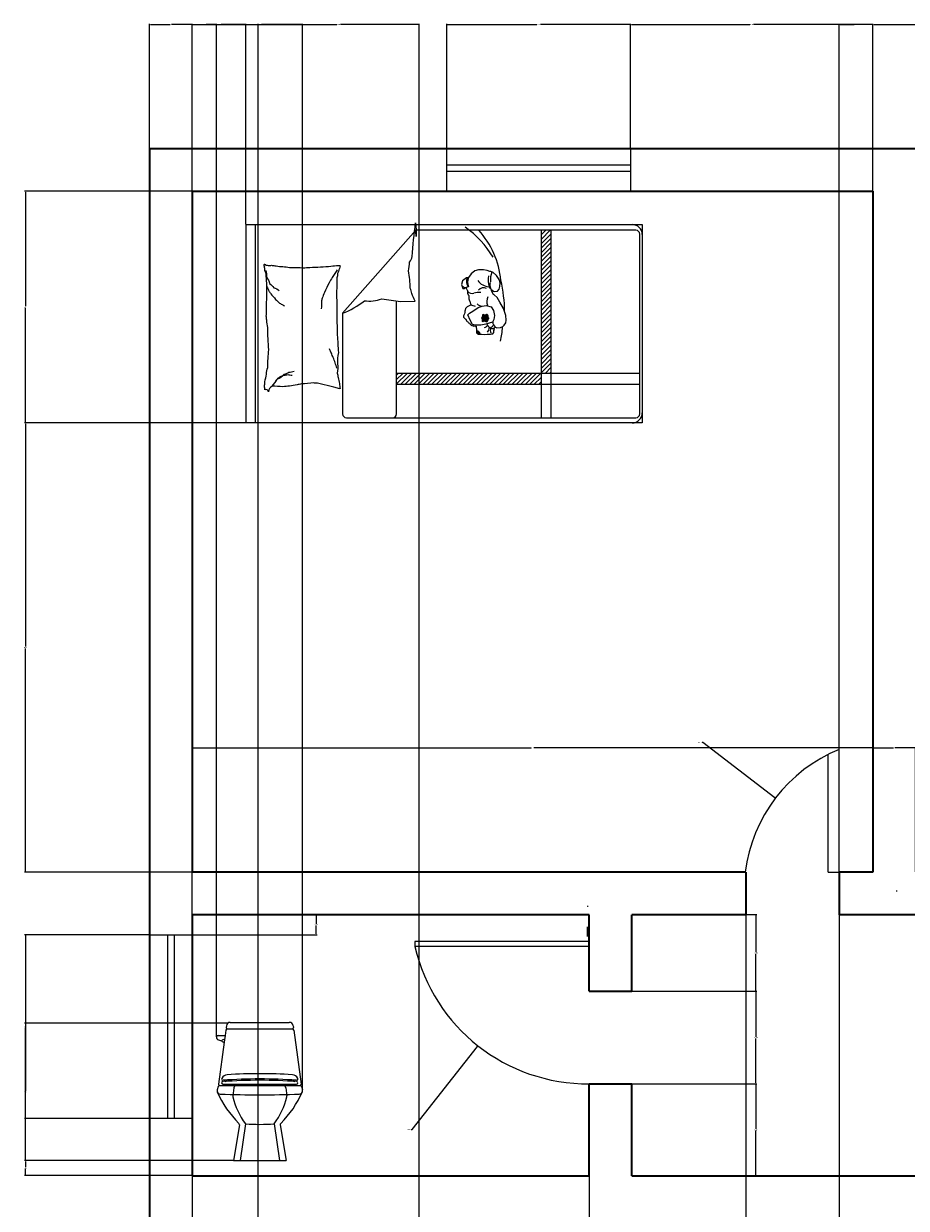
# Model space of a CAD drawing. Units: inches. Extents: x -20 to 351, y -512 to 63.
# Tile 4 of 5: x -20 to 166, y -188 to 63. Entities that reach past the tile are written whole.
import ezdxf

# ---------------------------------------------------------------- set-up
doc = ezdxf.new("R2010")
doc.units = ezdxf.units.IN
doc.header["$MEASUREMENT"] = 0
for name, color, linetype, lineweight in [('A-ANNO-DIMS', 2, 'Continuous', 18), ('A-DOOR', 3, 'Continuous', 18), ('A-FURN', 30, 'Continuous', 18), ('A-GLAZ', 4, 'Continuous', 18), ('A-WALL', 7, 'Continuous', 35), ('WC-Detail_dwgmodels.com', 31, 'Continuous', 13), ('WC-Outline_dwgmodels.com', 31, 'Continuous', 18)]:
    doc.layers.add(name, color=color, linetype=linetype, lineweight=lineweight)
doc.styles.get("Standard").update_dxf_attribs({"font": 'arial.ttf'})
doc.dimstyles.get("Standard").update_dxf_attribs({"dimtxt": 0.18, "dimasz": 0.18, "dimexe": 0.18, "dimexo": 0.0625, "dimgap": 0.09, "dimtad": 0, "dimtih": 1, "dimtoh": 1, "dimdec": 4, "dimzin": 0, "dimdsep": 46, "dimtxsty": 'Standard', "dimcen": 0.09, "dimadec": 0, "dimazin": 0, "dimtfac": 1, "dimtdec": 4, "dimtofl": 0, "dimtmove": 0, "dimatfit": 3, "dimfxl": 1, "dimtolj": 1, "dimtzin": 0, "dimarcsym": 0})
pattern_1 = [(135, (-420.77409, 493.76136), (-0.08072188, -0.08072188), [])]

# ---------------------------------------------------------------- blocks, each defined once
blk = doc.blocks.new('BED-SINGLE')
h = blk.add_hatch()
h.set_pattern_fill('ANSI31', color=256, scale=0.209657, angle=90, style=0)
h.set_pattern_definition([(225, (-28.8794, 49.6857), (-0.4706923, 0.4706923), [])])
h.paths.add_polyline_path([(62.56, 8.11), (62.56, 10.46), (31.92, 10.46), (31.92, 8.11)])
h.paths.add_polyline_path([(64.62, 10.46), (64.62, 40.74), (62.56, 40.74), (62.56, 10.46)])
h = blk.add_hatch()
h.set_pattern_fill('ANSI31', color=256, scale=0.913264, angle=90, style=0)
h.set_pattern_definition(pattern_1)
h.paths.add_polyline_path([(51.28, 22.35), (51.3, 22.58), (51.22, 22.8), (51.07, 22.92), (50.9, 22.92), (50.65, 22.81), (50.46, 22.77), (50.38, 22.84), (50.26, 22.89), (50.12, 22.84), (50.1, 22.73), (50.1, 22.6), (50.04, 22.43), (49.91, 22.22), (49.88, 22.16), (50.03, 21.91), (50.07, 21.8), (50.04, 21.63), (50.02, 21.51), (50.13, 21.39), (50.25, 21.43), (50.34, 21.55), (50.56, 21.53), (50.93, 21.38), (51.11, 21.41), (51.13, 21.53), (51.16, 21.62), (51.25, 21.7), (51.25, 21.79), (51.3, 21.95), (51.4, 22.06), (51.46, 22.11), (51.37, 22.18)])
h = blk.add_hatch()
h.set_pattern_fill('ANSI31', color=256, scale=0.913264, angle=90, style=0)
h.set_pattern_definition(pattern_1)
h.paths.add_polyline_path([(48.8, 19.38), (48.81, 19.17), (48.88, 18.99), (49.05, 18.85), (49.19, 18.79), (49.55, 18.75, 0.479357)])
for p, q in [((0, 41.93), (83.86, 41.93)), ((20.48, 23.17), (35.99, 40.74)), ((82.51, 40.74), (35.99, 40.74)), ((62.56, 1.08), (62.56, 40.74)), ((64.62, 1.08), (64.62, 40.74)), ((83.86, 41.93), (83.86, 0)), ((83.35, 1.92), (83.35, 39.9)), ((31.92, 1.92), (31.92, 25.76)), ((20.48, 23.17), (20.48, 1.92)), ((83.86, 0), (0, 0)), ((21.32, 1.08), (82.51, 1.08))]:
    blk.add_line(p, q)
for points in [[(0, 41.93), (0, 0)], [(2.1, 0), (2.1, 41.93)], [(49.88, 18.74), (50.44, 18.72), (51.09, 18.75), (51.78, 18.78), (51.99, 18.81), (52.24, 18.82), (52.5, 19.09), (52.51, 19.35), (52.46, 19.55), (52.59, 19.75), (52.54, 19.93), (52.68, 20.27), (52.85, 20.24), (53.09, 20.11), (53.92, 20.14), (54.4, 20.39), (54.7, 20.65), (55.03, 21.16), (55.11, 21.69), (54.99, 22.73), (54.51, 24.21), (53.78, 25.53), (53.17, 26.52), (52.53, 27.05), (52.38, 27.16), (51.98, 27.94), (51.97, 28.02), (52.04, 28.1), (52.44, 27.84), (52.72, 27.76), (53.28, 27.82), (53.58, 28.27), (53.78, 28.87), (53.81, 29.61), (53.61, 30.34), (53.08, 31.16), (52.32, 31.81), (51.86, 31.98), (51.61, 32), (51.05, 32.23), (50.29, 32.34), (49.27, 32.34), (48.48, 32.12), (47.69, 31.5), (47.1, 30.74), (46.7, 30.65), (45.83, 30.03), (45.63, 29.27), (45.94, 28.45), (46.23, 28.39), (46.51, 28.63), (46.59, 28.65), (46.7, 28.38), (46.79, 28.19), (46.84, 28.15), (46.88, 27.91), (46.94, 27.83), (46.9, 27.43), (47.08, 27.07), (47.21, 26.95), (47.22, 26.46), (47.16, 26.24), (47.34, 25.81), (47.42, 25.77), (47.46, 25.38), (47.62, 25.1), (47.53, 24.92), (47.25, 24.78), (46.82, 24.56), (46.52, 24.21), (46.42, 23.85), (46.36, 23.64), (46.33, 23.32), (46.29, 23.08), (46.15, 22.79), (46.09, 22.63), (46.1, 22.34), (46.39, 21.98), (46.55, 21.94), (46.69, 21.61), (46.82, 21.43), (46.98, 21.37), (47.06, 21.28), (47.13, 21.18), (47.37, 21.06), (47.42, 21.02), (47.42, 20.94), (47.65, 20.72), (47.76, 20.61), (47.94, 20.63), (48.13, 20.48), (48.29, 20.49), (48.59, 20.46), (48.72, 20.43), (48.78, 20.4), (48.76, 20.33), (48.74, 20.13), (48.82, 19.97), (48.83, 19.89), (48.79, 19.52), (48.81, 19.17), (48.88, 18.99), (49.05, 18.85), (49.19, 18.79), (49.73, 18.74), (49.88, 18.74)], [(47.98, 20.81), (47.46, 21.73), (46.99, 22.87), (47.37, 23.23), (48.03, 23.64), (49.19, 24.37), (50.01, 24.7), (50.89, 24.79), (51.92, 24.54), (52.4, 23.78), (52.6, 22.7), (52.51, 21.89), (52.18, 21.31), (50.82, 20.9), (49.74, 20.66), (48.6, 20.63), (47.98, 20.81)], [(49.88, 22.16), (50.03, 21.91), (50.07, 21.8), (50.04, 21.63), (50.02, 21.51), (50.13, 21.39), (50.25, 21.43), (50.34, 21.55), (50.56, 21.53), (50.93, 21.38), (51.11, 21.41), (51.13, 21.53), (51.16, 21.62), (51.25, 21.7), (51.25, 21.79), (51.3, 21.95), (51.4, 22.06), (51.46, 22.11), (51.37, 22.18), (51.28, 22.35), (51.3, 22.58), (51.22, 22.8), (51.07, 22.92), (50.9, 22.92), (50.65, 22.81), (50.46, 22.77), (50.38, 22.84), (50.26, 22.89), (50.12, 22.84), (50.1, 22.73), (50.1, 22.6), (50.04, 22.43), (49.91, 22.22), (49.88, 22.16)], [(83.35, 10.46), (31.92, 10.46)], [(83.35, 8.11), (31.92, 8.11)]]:
    blk.add_lwpolyline(points)
for points in [[(35.81, 25.72, 0.027362), (35.12, 27.33, 0.040834), (34.81, 28.47, 0.038441), (34.42, 32.14, 0.076528), (34.64, 34, 0.103649), (35.24, 35.15, -0.018778), (35.94, 42.28, -0.024037), (36.09, 39.44, -0.052315), (35.99, 40.74)], [(5.6, 7.76, 0.263368), (4.81, 6.59, 0.494818), (4.03, 6.97, 0.049225), (3.96, 7.71, 0.036831), (4.03, 8.71, 0.031893), (4.37, 10.3, -0.035782), (4.66, 11.72, -0.032941), (4.91, 15.48, -0.026564), (4.66, 20.14, -0.017905), (4.44, 21.72, 0.033397), (4.34, 22.56, 0.03204), (4.37, 24.12, -0.018442), (4.5, 26.82, -0.010837), (4.47, 29.53, -0.014624), (4.34, 31.54, -0.111249), (4.04, 32.49, 0.153708), (3.87, 33.19, 0.076444), (3.94, 33.51, 0.215512), (4.03, 33.59, 0.585858), (4.16, 33.48, -0.363489), (4.26, 33.27, -0.191716), (4.75, 33.27, 0.129675), (5.45, 33.35, 0.01735), (6.15, 33.23, -0.019326), (6.78, 33.12, -0.018818), (9.65, 32.84, -0.021828), (12.13, 32.8, -0.006204), (13.55, 32.86, -0.001963), (18.04, 33.12, -0.028341), (19.55, 33.29, 0.117014), (19.92, 33.27, 0.36606), (19.96, 33.21, 0.03973), (19.84, 32.64, 0.048309), (19.62, 32.07, -0.062981), (19.45, 31.62, -0.04058), (19.31, 30.64, -0.014345), (19.22, 27.84, -0.005484), (19.25, 22.58, -0.007153), (19.37, 18.55, -0.008762), (19.49, 16.76, 0.008153), (19.61, 14.85, 0.06251), (19.42, 12.45, -0.078669), (19.34, 10.54, -0.047825), (19.54, 9.6, 0.034494), (19.84, 8.31, 0.023571), (19.97, 7.25, 0.510228), (19.92, 7.21), (18.66, 7.52), (15.2, 8.39, -0.073041), (14.38, 8.47, -0.023305), (11.82, 8.23, -0.018299), (10.86, 8.06, 0.01097), (9.27, 7.75, 0.042281), (7.83, 7.63, 0.027201), (5.59, 7.75)], [(4.26, 32.24, -0.088153), (4.41, 30.79, -0.088153), (5.05, 29.48, -0.077547), (5.96, 28.58, -0.077547), (7.1, 27.99)], [(19.37, 32.4, -0.016108), (18.27, 30.77, -0.024599), (17.64, 29.64, -0.009477), (16.66, 27.59, -0.015937), (16.15, 26.34, -0.072521), (16, 25.65, -0.033339), (15.99, 24.13)], [(4.5, 28.8, -0.027842), (4.95, 27.81, -0.048685), (5.29, 27.28, -0.023666), (6.31, 26.11, -0.031223), (7.18, 25.31, -0.046801), (7.5, 25.1, -0.023191), (8.2, 24.76)], [(20.48, 23.17, 0.085272), (25.1, 25.83, 0.124044), (28.77, 26.21), (32.77, 25.64), (35.81, 25.72)], [(19.31, 11.55, -0.009729), (18.93, 12.7, -0.009729), (18.51, 13.82, -0.007971), (18.13, 14.74, -0.007971), (17.72, 15.64)], [(5.6, 7.75, 0.077379), (6.66, 9.21, 0.077379), (8.12, 10.28, 0.047525), (9.15, 10.7, 0.047525), (10.25, 10.91)], [(6.27, 8.86, 0.05369), (6.82, 9.46, 0.070312), (7.33, 9.8, 0.015448), (7.69, 9.96, 0.013244), (8.12, 10.11, 0.082127), (8.88, 10.24, 0.064164), (9.85, 10.11)]]:
    blk.add_lwpolyline(points, format="xyb")
for centre, radius, start, end in [((33.6, 23.46), 22.04, 31.7708, 54.3375), ((35.62, 28.39), 18.42, 5.4641, 42.1092), ((81.77, 39.84), 2.1, 0, 90), ((82.51, 39.9), 0.839, 0, 90), ((48.38, 29.88), 1.69, 151.149, 221.3836), ((49.8, 29.77), 2.87, 160.3319, 200.5181), ((51.72, 32.02), 3.26, 215.9219, 265.4055), ((57.03, 30.22), 5.75, 171.0084, 194.554), ((56.22, 30.19), 4.47, 157.6837, 184.5902), ((27.13, 23.57), 27.62, 359.7962, 13.7616), ((46.52, 29.27), 0.673, 218.3031, 258.9374), ((47.06, 28.21), 0.555, 83.9542, 141.018), ((47.86, 28.52), 1.15, 217.108, 288.2435), ((49.63, 21.97), 5.63, 89.2848, 104.5089), ((50.34, 27.01), 1.56, 67.4286, 136.0363), ((50.26, 27.3), 1.9, 23.4063, 50.8909), ((54.62, 29.31), 2.97, 172.9692, 196.7988), ((50.11, 26.41), 1.71, 226.7949, 266.7156), ((52.75, 25.69), 1.78, 147.515, 207.2356), ((50.24, 30.81), 6.38, 245.3415, 254.4913), ((50.34, 21.04), 0.905, 279.9605, 331.843), ((52.62, 21.72), 1.86, 210.5886, 253.4912), ((50.37, 20.09), 1.16, 309.7451, 1.7337), ((51.62, 20.94), 0.779, 295.2148, 339.8011), ((52.13, 20.47), 0.53, 266.1994, 319.0666), ((53.63, 21.39), 1.39, 182.1498, 236.1783), ((12.56, 24.85), 42.04, 349.6217, 353.7472), ((48.92, 18.76), 0.631, 359.0987, 101.5429), ((53.53, 19.57), 1.79, 164.8422, 197.2397), ((21.32, 1.92), 0.839, 180, 270), ((31.08, 1.92), 0.839, 270, 0), ((81.77, 2.1), 2.1, 270, 0), ((82.51, 1.92), 0.839, 270, 0)]:
    blk.add_arc(centre, radius, start, end)
blk = doc.blocks.new('*D11')
at = {"layer": 'A-ANNO-DIMS', "color": 0, "lineweight": -2, "transparency": 16777216}
for p, q in [((69.14, 36.3), (69.14, 62.67)), ((108.03, 36.3), (108.03, 62.67)), ((69.32, 62.49), (88.19, 62.49)), ((107.85, 62.49), (88.98, 62.49))]:
    blk.add_line(p, q, dxfattribs=at)
at = {"layer": 'A-ANNO-DIMS', "color": 0, "transparency": 16777216}
for points in [[(69.32, 62.52), (69.32, 62.46), (69.14, 62.49)], [(107.85, 62.52), (107.85, 62.46), (108.03, 62.49)]]:
    blk.add_solid(points, dxfattribs=at)
at = {"layer": 'Defpoints', "color": 0, "transparency": 16777216}
for p in [(108.03, 62.49), (69.14, 36.24), (108.03, 36.24)]:
    blk.add_point(p, dxfattribs=at)
at = {"layer": 'A-ANNO-DIMS', "color": 0, "transparency": 16777216, "insert": (88.59, 62.49), "char_height": 0.18, "attachment_point": 5}
blk.add_mtext('\\A1;38.88', dxfattribs=at)
blk = doc.blocks.new('*D12')
at = {"layer": 'A-ANNO-DIMS', "color": 0, "lineweight": -2, "transparency": 16777216}
for p, q in [((108.03, 36.3), (108.03, 62.67)), ((159.28, 27.3), (159.28, 62.67)), ((108.21, 62.49), (133.26, 62.49)), ((159.1, 62.49), (134.05, 62.49))]:
    blk.add_line(p, q, dxfattribs=at)
at = {"layer": 'A-ANNO-DIMS', "color": 0, "transparency": 16777216}
for points in [[(108.21, 62.52), (108.21, 62.46), (108.03, 62.49)], [(159.1, 62.52), (159.1, 62.46), (159.28, 62.49)]]:
    blk.add_solid(points, dxfattribs=at)
at = {"layer": 'Defpoints', "color": 0, "transparency": 16777216}
for p in [(159.28, 62.49), (108.03, 36.24), (159.28, 27.24)]:
    blk.add_point(p, dxfattribs=at)
at = {"layer": 'A-ANNO-DIMS', "color": 0, "transparency": 16777216, "insert": (133.66, 62.49), "char_height": 0.18, "attachment_point": 5}
blk.add_mtext('\\A1;51.26', dxfattribs=at)
blk = doc.blocks.new('*D13')
at = {"layer": 'A-ANNO-DIMS', "color": 0, "lineweight": -2, "transparency": 16777216}
for p, q in [((159.28, 27.3), (159.28, 62.67)), ((224.21, 36.3), (224.21, 62.67)), ((159.46, 62.49), (191.35, 62.49)), ((224.03, 62.49), (192.14, 62.49))]:
    blk.add_line(p, q, dxfattribs=at)
at = {"layer": 'A-ANNO-DIMS', "color": 0, "transparency": 16777216}
for points in [[(159.46, 62.52), (159.46, 62.46), (159.28, 62.49)], [(224.03, 62.52), (224.03, 62.46), (224.21, 62.49)]]:
    blk.add_solid(points, dxfattribs=at)
at = {"layer": 'Defpoints', "color": 0, "transparency": 16777216}
for p in [(224.21, 62.49), (224.21, 36.24), (159.28, 27.24)]:
    blk.add_point(p, dxfattribs=at)
at = {"layer": 'A-ANNO-DIMS', "color": 0, "transparency": 16777216, "insert": (191.74, 62.49), "char_height": 0.18, "attachment_point": 5}
blk.add_mtext('\\A1;64.92', dxfattribs=at)
blk = doc.blocks.new('*D15')
at = {"layer": 'A-ANNO-DIMS', "color": 0, "lineweight": -2, "transparency": 16777216}
for p, q in [((15.35, -125.76), (41.71, -125.76)), ((41.53, -125.94), (41.53, -127.71)), ((15.35, -130.02), (41.71, -130.02)), ((41.53, -129.84), (41.53, -128.07))]:
    blk.add_line(p, q, dxfattribs=at)
at = {"layer": 'A-ANNO-DIMS', "color": 0, "transparency": 16777216}
for points in [[(41.5, -125.94), (41.56, -125.94), (41.53, -125.76)], [(41.5, -129.84), (41.56, -129.84), (41.53, -130.02)]]:
    blk.add_solid(points, dxfattribs=at)
at = {"layer": 'Defpoints', "color": 0, "transparency": 16777216}
for p in [(15.28, -125.76), (15.28, -130.02), (41.53, -130.02)]:
    blk.add_point(p, dxfattribs=at)
at = {"layer": 'A-ANNO-DIMS', "color": 0, "transparency": 16777216, "insert": (41.53, -127.89), "char_height": 0.18, "attachment_point": 5}
blk.add_mtext('\\A1;4.256', dxfattribs=at)
blk = doc.blocks.new('*D16')
at = {"layer": 'A-ANNO-DIMS', "color": 0, "lineweight": -2, "transparency": 16777216}
for p, q in [((6.22, -130.02), (-20.15, -130.02)), ((-19.97, -130.2), (-19.97, -149.28)), ((-19.97, -168.72), (-19.97, -149.64)), ((6.22, -168.9), (-20.15, -168.9))]:
    blk.add_line(p, q, dxfattribs=at)
at = {"layer": 'A-ANNO-DIMS', "color": 0, "transparency": 16777216}
for points in [[(-20, -130.2), (-19.94, -130.2), (-19.97, -130.02)], [(-20, -168.72), (-19.94, -168.72), (-19.97, -168.9)]]:
    blk.add_solid(points, dxfattribs=at)
at = {"layer": 'Defpoints', "color": 0, "transparency": 16777216}
for p in [(6.28, -130.02), (-19.97, -168.9), (6.28, -168.9)]:
    blk.add_point(p, dxfattribs=at)
at = {"layer": 'A-ANNO-DIMS', "color": 0, "transparency": 16777216, "insert": (-19.97, -149.46), "char_height": 0.18, "attachment_point": 5}
blk.add_mtext('\\A1;38.88', dxfattribs=at)
blk = doc.blocks.new('*D31')
at = {"layer": 'A-ANNO-DIMS', "color": 0, "lineweight": -2, "transparency": 16777216}
for p, q in [((15.28, -116.7), (15.28, -90.33)), ((15.46, -90.51), (87, -90.51)), ((159.1, -90.51), (87.56, -90.51)), ((159.28, -116.7), (159.28, -90.33))]:
    blk.add_line(p, q, dxfattribs=at)
at = {"layer": 'A-ANNO-DIMS', "color": 0, "transparency": 16777216}
for points in [[(15.46, -90.48), (15.46, -90.54), (15.28, -90.51)], [(159.1, -90.48), (159.1, -90.54), (159.28, -90.51)]]:
    blk.add_solid(points, dxfattribs=at)
at = {"layer": 'Defpoints', "color": 0, "transparency": 16777216}
for p in [(159.28, -90.51), (15.28, -116.76), (159.28, -116.76)]:
    blk.add_point(p, dxfattribs=at)
at = {"layer": 'A-ANNO-DIMS', "color": 0, "transparency": 16777216, "insert": (87.28, -90.51), "char_height": 0.18, "attachment_point": 5}
blk.add_mtext('\\A1;144', dxfattribs=at)
blk = doc.blocks.new('*D32')
at = {"layer": 'A-ANNO-DIMS', "color": 0, "lineweight": -2, "transparency": 16777216}
for p, q in [((26.56, -21.75), (-20.15, -21.75)), ((-19.97, -21.93), (-19.97, -69.08)), ((-19.97, -116.58), (-19.97, -69.44)), ((15.22, -116.76), (-20.15, -116.76))]:
    blk.add_line(p, q, dxfattribs=at)
at = {"layer": 'A-ANNO-DIMS', "color": 0, "transparency": 16777216}
for points in [[(-20, -21.93), (-19.94, -21.93), (-19.97, -21.75)], [(-20, -116.58), (-19.94, -116.58), (-19.97, -116.76)]]:
    blk.add_solid(points, dxfattribs=at)
at = {"layer": 'Defpoints', "color": 0, "transparency": 16777216}
for p in [(26.62, -21.75), (-19.97, -116.76), (15.28, -116.76)]:
    blk.add_point(p, dxfattribs=at)
at = {"layer": 'A-ANNO-DIMS', "color": 0, "transparency": 16777216, "insert": (-19.97, -69.26), "char_height": 0.18, "attachment_point": 5}
blk.add_mtext('\\A1;95.01', dxfattribs=at)
blk = doc.blocks.new('*D33')
at = {"layer": 'A-ANNO-DIMS', "color": 0, "lineweight": -2, "transparency": 16777216}
for p, q in [((159.28, -116.7), (159.28, -90.33)), ((159.46, -90.51), (163.64, -90.51)), ((168.1, -90.51), (163.93, -90.51)), ((168.28, -116.7), (168.28, -90.33))]:
    blk.add_line(p, q, dxfattribs=at)
at = {"layer": 'A-ANNO-DIMS', "color": 0, "transparency": 16777216}
for points in [[(159.46, -90.48), (159.46, -90.54), (159.28, -90.51)], [(168.1, -90.48), (168.1, -90.54), (168.28, -90.51)]]:
    blk.add_solid(points, dxfattribs=at)
at = {"layer": 'Defpoints', "color": 0, "transparency": 16777216}
for p in [(168.28, -90.51), (159.28, -116.76), (168.28, -116.76)]:
    blk.add_point(p, dxfattribs=at)
at = {"layer": 'A-ANNO-DIMS', "color": 0, "transparency": 16777216, "insert": (163.78, -90.51), "char_height": 0.18, "attachment_point": 5}
blk.add_mtext('\\A1;9', dxfattribs=at)
blk = doc.blocks.new('*D34')
at = {"layer": 'A-ANNO-DIMS', "color": 0, "lineweight": -2, "transparency": 16777216}
for p, q in [((6.28, -129.96), (6.28, 62.67)), ((15.28, -129.96), (15.28, 62.67)), ((6.46, 62.49), (10.64, 62.49)), ((15.1, 62.49), (10.93, 62.49))]:
    blk.add_line(p, q, dxfattribs=at)
at = {"layer": 'A-ANNO-DIMS', "color": 0, "transparency": 16777216}
for points in [[(6.46, 62.52), (6.46, 62.46), (6.28, 62.49)], [(15.1, 62.52), (15.1, 62.46), (15.28, 62.49)]]:
    blk.add_solid(points, dxfattribs=at)
at = {"layer": 'Defpoints', "color": 0, "transparency": 16777216}
for p in [(15.28, 62.49), (6.28, -130.02), (15.28, -130.02)]:
    blk.add_point(p, dxfattribs=at)
at = {"layer": 'A-ANNO-DIMS', "color": 0, "transparency": 16777216, "insert": (10.78, 62.49), "char_height": 0.18, "attachment_point": 5}
blk.add_mtext('\\A1;9', dxfattribs=at)
blk = doc.blocks.new('*D35')
at = {"layer": 'A-ANNO-DIMS', "color": 0, "lineweight": -2, "transparency": 16777216}
for p, q in [((15.28, -181.03), (15.28, -512.19)), ((99.28, -181.03), (99.28, -512.19)), ((15.46, -512.01), (57.07, -512.01)), ((99.1, -512.01), (57.5, -512.01))]:
    blk.add_line(p, q, dxfattribs=at)
at = {"layer": 'A-ANNO-DIMS', "color": 0, "transparency": 16777216}
for points in [[(15.46, -511.98), (15.46, -512.04), (15.28, -512.01)], [(99.1, -511.98), (99.1, -512.04), (99.28, -512.01)]]:
    blk.add_solid(points, dxfattribs=at)
at = {"layer": 'Defpoints', "color": 0, "transparency": 16777216}
for p in [(15.28, -180.96), (99.28, -180.96), (99.28, -512.01)]:
    blk.add_point(p, dxfattribs=at)
at = {"layer": 'A-ANNO-DIMS', "color": 0, "transparency": 16777216, "insert": (57.28, -512.01), "char_height": 0.18, "attachment_point": 5}
blk.add_mtext('\\A1;84', dxfattribs=at)
blk = doc.blocks.new('*D36')
at = {"layer": 'A-ANNO-DIMS', "color": 0, "lineweight": -2, "transparency": 16777216}
for p, q in [((108.35, -161.54), (134.71, -161.54)), ((134.53, -161.72), (134.53, -171.07)), ((134.53, -180.78), (134.53, -171.43)), ((108.35, -180.96), (134.71, -180.96))]:
    blk.add_line(p, q, dxfattribs=at)
at = {"layer": 'A-ANNO-DIMS', "color": 0, "transparency": 16777216}
for points in [[(134.5, -161.72), (134.56, -161.72), (134.53, -161.54)], [(134.5, -180.78), (134.56, -180.78), (134.53, -180.96)]]:
    blk.add_solid(points, dxfattribs=at)
at = {"layer": 'Defpoints', "color": 0, "transparency": 16777216}
for p in [(108.28, -161.54), (108.28, -180.96), (134.53, -180.96)]:
    blk.add_point(p, dxfattribs=at)
at = {"layer": 'A-ANNO-DIMS', "color": 0, "transparency": 16777216, "insert": (134.53, -171.25), "char_height": 0.18, "attachment_point": 5}
blk.add_mtext('\\A1;19.427', dxfattribs=at)
blk = doc.blocks.new('*D39')
at = {"layer": 'A-ANNO-DIMS', "color": 0, "lineweight": -2, "transparency": 16777216}
for p, q in [((152.16, -116.7), (152.16, 62.67)), ((159.28, -116.7), (159.28, 62.67)), ((152.34, 62.49), (155.33, 62.49)), ((159.1, 62.49), (156.12, 62.49))]:
    blk.add_line(p, q, dxfattribs=at)
at = {"layer": 'A-ANNO-DIMS', "color": 0, "transparency": 16777216}
for points in [[(152.34, 62.52), (152.34, 62.46), (152.16, 62.49)], [(159.1, 62.52), (159.1, 62.46), (159.28, 62.49)]]:
    blk.add_solid(points, dxfattribs=at)
at = {"layer": 'Defpoints', "color": 0, "transparency": 16777216}
for p in [(152.16, 62.49), (152.16, -116.76), (159.28, -116.76)]:
    blk.add_point(p, dxfattribs=at)
at = {"layer": 'A-ANNO-DIMS', "color": 0, "transparency": 16777216, "insert": (155.72, 62.49), "char_height": 0.18, "attachment_point": 5}
blk.add_mtext('\\A1;7.124', dxfattribs=at)
blk = doc.blocks.new('*D40')
at = {"layer": 'A-ANNO-DIMS', "color": 0, "lineweight": -2, "transparency": 16777216}
for p, q in [((132.43, -125.83), (132.43, -512.19)), ((152.16, -125.83), (152.16, -512.19)), ((132.61, -512.01), (141.84, -512.01)), ((151.98, -512.01), (142.75, -512.01))]:
    blk.add_line(p, q, dxfattribs=at)
at = {"layer": 'A-ANNO-DIMS', "color": 0, "transparency": 16777216}
for points in [[(132.61, -511.98), (132.61, -512.04), (132.43, -512.01)], [(151.98, -511.98), (151.98, -512.04), (152.16, -512.01)]]:
    blk.add_solid(points, dxfattribs=at)
at = {"layer": 'Defpoints', "color": 0, "transparency": 16777216}
for p in [(132.43, -125.76), (152.16, -125.76), (132.43, -512.01)]:
    blk.add_point(p, dxfattribs=at)
at = {"layer": 'A-ANNO-DIMS', "color": 0, "transparency": 16777216, "insert": (142.3, -512.01), "char_height": 0.18, "attachment_point": 5}
blk.add_mtext('\\A1;19.727', dxfattribs=at)
blk = doc.blocks.new('*D43')
at = {"layer": 'A-ANNO-DIMS', "color": 0, "lineweight": -2, "transparency": 16777216}
for p, q in [((108.35, -125.76), (134.71, -125.76)), ((134.53, -125.94), (134.53, -133.69)), ((134.53, -141.79), (134.53, -134.05)), ((108.35, -141.97), (134.71, -141.97))]:
    blk.add_line(p, q, dxfattribs=at)
at = {"layer": 'A-ANNO-DIMS', "color": 0, "transparency": 16777216}
for points in [[(134.5, -125.94), (134.56, -125.94), (134.53, -125.76)], [(134.5, -141.79), (134.56, -141.79), (134.53, -141.97)]]:
    blk.add_solid(points, dxfattribs=at)
at = {"layer": 'Defpoints', "color": 0, "transparency": 16777216}
for p in [(108.28, -125.76), (108.28, -141.97), (134.53, -141.97)]:
    blk.add_point(p, dxfattribs=at)
at = {"layer": 'A-ANNO-DIMS', "color": 0, "transparency": 16777216, "insert": (134.53, -133.87), "char_height": 0.18, "attachment_point": 5}
blk.add_mtext('\\A1;16.208', dxfattribs=at)
blk = doc.blocks.new('*D44')
at = {"layer": 'A-ANNO-DIMS', "color": 0, "lineweight": -2, "transparency": 16777216}
for p, q in [((108.35, -141.97), (134.71, -141.97)), ((134.53, -142.15), (134.53, -151.57)), ((134.53, -161.36), (134.53, -151.94)), ((108.35, -161.54), (134.71, -161.54))]:
    blk.add_line(p, q, dxfattribs=at)
at = {"layer": 'A-ANNO-DIMS', "color": 0, "transparency": 16777216}
for points in [[(134.5, -142.15), (134.56, -142.15), (134.53, -141.97)], [(134.5, -161.36), (134.56, -161.36), (134.53, -161.54)]]:
    blk.add_solid(points, dxfattribs=at)
at = {"layer": 'Defpoints', "color": 0, "transparency": 16777216}
for p in [(108.28, -141.97), (108.28, -161.54), (134.53, -161.54)]:
    blk.add_point(p, dxfattribs=at)
at = {"layer": 'A-ANNO-DIMS', "color": 0, "transparency": 16777216, "insert": (134.53, -151.76), "char_height": 0.18, "attachment_point": 5}
blk.add_mtext('\\A1;19.565', dxfattribs=at)
blk = doc.blocks.new('*D51')
at = {"layer": 'A-ANNO-DIMS', "color": 0, "lineweight": -2, "transparency": 16777216}
for p, q in [((29.23, -468.97), (29.23, 62.67)), ((63.28, -476.7), (63.28, 62.67)), ((29.41, 62.49), (45.86, 62.49)), ((63.1, 62.49), (46.65, 62.49))]:
    blk.add_line(p, q, dxfattribs=at)
at = {"layer": 'A-ANNO-DIMS', "color": 0, "transparency": 16777216}
for points in [[(29.41, 62.52), (29.41, 62.46), (29.23, 62.49)], [(63.1, 62.52), (63.1, 62.46), (63.28, 62.49)]]:
    blk.add_solid(points, dxfattribs=at)
at = {"layer": 'Defpoints', "color": 0, "transparency": 16777216}
for p in [(63.28, 62.49), (29.23, -469.03), (63.28, -476.76)]:
    blk.add_point(p, dxfattribs=at)
at = {"layer": 'A-ANNO-DIMS', "color": 0, "transparency": 16777216, "insert": (46.26, 62.49), "char_height": 0.18, "attachment_point": 5}
blk.add_mtext('\\A1;34.06', dxfattribs=at)
blk = doc.blocks.new('*D67')
at = {"layer": 'A-ANNO-DIMS', "color": 0, "lineweight": -2, "transparency": 16777216}
for p, q in [((15.28, 27.3), (15.28, 62.67)), ((26.62, 20.24), (26.62, 62.67)), ((15.46, 62.49), (20.5, 62.49)), ((26.44, 62.49), (21.41, 62.49))]:
    blk.add_line(p, q, dxfattribs=at)
at = {"layer": 'A-ANNO-DIMS', "color": 0, "transparency": 16777216}
for points in [[(15.46, 62.52), (15.46, 62.46), (15.28, 62.49)], [(26.44, 62.52), (26.44, 62.46), (26.62, 62.49)]]:
    blk.add_solid(points, dxfattribs=at)
at = {"layer": 'Defpoints', "color": 0, "transparency": 16777216}
for p in [(26.62, 62.49), (15.28, 27.24), (26.62, 20.18)]:
    blk.add_point(p, dxfattribs=at)
at = {"layer": 'A-ANNO-DIMS', "color": 0, "transparency": 16777216, "insert": (20.95, 62.49), "char_height": 0.18, "attachment_point": 5}
blk.add_mtext('\\A1;11.334', dxfattribs=at)
blk = doc.blocks.new('*D68')
at = {"layer": 'A-ANNO-DIMS', "color": 0, "lineweight": -2, "transparency": 16777216}
for p, q in [((15.22, 27.24), (-20.15, 27.24)), ((-19.97, 27.06), (-19.97, 2.92)), ((-19.97, -21.57), (-19.97, 2.56)), ((26.56, -21.75), (-20.15, -21.75))]:
    blk.add_line(p, q, dxfattribs=at)
at = {"layer": 'A-ANNO-DIMS', "color": 0, "transparency": 16777216}
for points in [[(-20, 27.06), (-19.94, 27.06), (-19.97, 27.24)], [(-20, -21.57), (-19.94, -21.57), (-19.97, -21.75)]]:
    blk.add_solid(points, dxfattribs=at)
at = {"layer": 'Defpoints', "color": 0, "transparency": 16777216}
for p in [(15.28, 27.24), (-19.97, -21.75), (26.62, -21.75)]:
    blk.add_point(p, dxfattribs=at)
at = {"layer": 'A-ANNO-DIMS', "color": 0, "transparency": 16777216, "insert": (-19.97, 2.74), "char_height": 0.18, "attachment_point": 5}
blk.add_mtext('\\A1;48.99', dxfattribs=at)
blk = doc.blocks.new('*D70')
at = {"layer": 'A-ANNO-DIMS', "color": 0, "lineweight": -2, "transparency": 16777216}
for p, q in [((15.28, -180.9), (15.28, 62.67)), ((20.42, -151.6), (20.42, 62.67)), ((15.46, 62.49), (17.46, 62.49)), ((20.24, 62.49), (18.24, 62.49))]:
    blk.add_line(p, q, dxfattribs=at)
at = {"layer": 'A-ANNO-DIMS', "color": 0, "transparency": 16777216}
for points in [[(15.46, 62.52), (15.46, 62.46), (15.28, 62.49)], [(20.24, 62.52), (20.24, 62.46), (20.42, 62.49)]]:
    blk.add_solid(points, dxfattribs=at)
at = {"layer": 'Defpoints', "color": 0, "transparency": 16777216}
for p in [(20.42, 62.49), (20.42, -151.67), (15.28, -180.96)]:
    blk.add_point(p, dxfattribs=at)
at = {"layer": 'A-ANNO-DIMS', "color": 0, "transparency": 16777216, "insert": (17.85, 62.49), "char_height": 0.18, "attachment_point": 5}
blk.add_mtext('\\A1;5.133', dxfattribs=at)
blk = doc.blocks.new('*D71')
at = {"layer": 'A-ANNO-DIMS', "color": 0, "lineweight": -2, "transparency": 16777216}
for p, q in [((23.97, -177.78), (-20.15, -177.78)), ((-19.97, -177.96), (-19.97, -179.19)), ((-19.97, -180.78), (-19.97, -179.55)), ((15.22, -180.96), (-20.15, -180.96))]:
    blk.add_line(p, q, dxfattribs=at)
at = {"layer": 'A-ANNO-DIMS', "color": 0, "transparency": 16777216}
for points in [[(-20, -177.96), (-19.94, -177.96), (-19.97, -177.78)], [(-20, -180.78), (-19.94, -180.78), (-19.97, -180.96)]]:
    blk.add_solid(points, dxfattribs=at)
at = {"layer": 'Defpoints', "color": 0, "transparency": 16777216}
for p in [(-19.97, -177.78), (24.03, -177.78), (15.28, -180.96)]:
    blk.add_point(p, dxfattribs=at)
at = {"layer": 'A-ANNO-DIMS', "color": 0, "transparency": 16777216, "insert": (-19.97, -179.37), "char_height": 0.18, "attachment_point": 5}
blk.add_mtext('\\A1;3.19', dxfattribs=at)
blk = doc.blocks.new('*D72')
at = {"layer": 'A-ANNO-DIMS', "color": 0, "lineweight": -2, "transparency": 16777216}
for p, q in [((22.76, -148.74), (-20.15, -148.74)), ((-19.97, -148.92), (-19.97, -163.08)), ((-19.97, -177.6), (-19.97, -163.44)), ((23.97, -177.78), (-20.15, -177.78))]:
    blk.add_line(p, q, dxfattribs=at)
at = {"layer": 'A-ANNO-DIMS', "color": 0, "transparency": 16777216}
for points in [[(-20, -148.92), (-19.94, -148.92), (-19.97, -148.74)], [(-20, -177.6), (-19.94, -177.6), (-19.97, -177.78)]]:
    blk.add_solid(points, dxfattribs=at)
at = {"layer": 'Defpoints', "color": 0, "transparency": 16777216}
for p in [(22.82, -148.74), (-19.97, -177.78), (24.03, -177.78)]:
    blk.add_point(p, dxfattribs=at)
at = {"layer": 'A-ANNO-DIMS', "color": 0, "transparency": 16777216, "insert": (-19.97, -163.26), "char_height": 0.18, "attachment_point": 5}
blk.add_mtext('\\A1;29.035', dxfattribs=at)
blk = doc.blocks.new('*D73')
at = {"layer": 'A-ANNO-DIMS', "color": 0, "lineweight": -2, "transparency": 16777216}
for p, q in [((20.42, -151.6), (20.42, 62.67)), ((38.65, -162.97), (38.65, 62.67)), ((20.6, 62.49), (29.08, 62.49)), ((38.47, 62.49), (29.99, 62.49))]:
    blk.add_line(p, q, dxfattribs=at)
at = {"layer": 'A-ANNO-DIMS', "color": 0, "transparency": 16777216}
for points in [[(20.6, 62.52), (20.6, 62.46), (20.42, 62.49)], [(38.47, 62.52), (38.47, 62.46), (38.65, 62.49)]]:
    blk.add_solid(points, dxfattribs=at)
at = {"layer": 'Defpoints', "color": 0, "transparency": 16777216}
for p in [(38.65, 62.49), (20.42, -151.67), (38.65, -163.03)]:
    blk.add_point(p, dxfattribs=at)
at = {"layer": 'A-ANNO-DIMS', "color": 0, "transparency": 16777216, "insert": (29.53, 62.49), "char_height": 0.18, "attachment_point": 5}
blk.add_mtext('\\A1;18.234', dxfattribs=at)
blk = doc.blocks.new('*D76')
at = {"layer": 'A-ANNO-DIMS', "color": 0, "lineweight": -2, "transparency": 16777216}
for p, q in [((123.14, -89.31), (123.32, -89.31)), ((123.32, -89.31), (138.55, -100.98)), ((164.23, -120.72), (164.41, -120.72)), ((164.32, -120.81), (164.32, -120.63))]:
    blk.add_line(p, q, dxfattribs=at)
at = {"layer": 'A-ANNO-DIMS', "color": 0, "transparency": 16777216}
blk.add_solid([(138.57, -100.95), (138.53, -101), (138.69, -101.09)], dxfattribs=at)
at = {"layer": 'Defpoints', "color": 0, "transparency": 16777216}
for p in [(138.69, -101.09), (164.32, -120.72)]:
    blk.add_point(p, dxfattribs=at)
at = {"layer": 'A-ANNO-DIMS', "color": 0, "transparency": 16777216, "insert": (122.66, -89.31), "char_height": 0.18, "attachment_point": 5}
blk.add_mtext('\\A1;R32.28', dxfattribs=at)
blk = doc.blocks.new('*D78')
at = {"layer": 'A-ANNO-DIMS', "color": 0, "lineweight": -2, "transparency": 16777216}
for p, q in [((98.9, -123.97), (99.08, -123.97)), ((98.99, -124.06), (98.99, -123.88)), ((61.8, -171.2), (75.64, -153.63)), ((61.62, -171.2), (61.8, -171.2))]:
    blk.add_line(p, q, dxfattribs=at)
at = {"layer": 'A-ANNO-DIMS', "color": 0, "transparency": 16777216}
blk.add_solid([(75.61, -153.61), (75.66, -153.65), (75.75, -153.49)], dxfattribs=at)
at = {"layer": 'Defpoints', "color": 0, "transparency": 16777216}
for p in [(98.99, -123.97), (75.75, -153.49)]:
    blk.add_point(p, dxfattribs=at)
at = {"layer": 'A-ANNO-DIMS', "color": 0, "transparency": 16777216, "insert": (61.14, -171.2), "char_height": 0.18, "attachment_point": 5}
blk.add_mtext('\\A1;R37.57', dxfattribs=at)

msp = doc.modelspace()

# ---------------------------------------------------------------- linework, layer by layer
at = {"layer": 'A-DOOR'}
for p, q in [((149.7902, -116.7646), (149.7902, -91.8924)), ((152.1609, -116.7646), (152.1609, -90.8152)), ((149.7902, -116.7646), (152.1609, -116.7646)), ((152.1609, -116.7646), (152.1609, -116.7646)), ((98.8637, -128.3681), (98.8637, -130.3681)), ((99.2844, -131.4137), (62.4001, -131.4137)), ((62.4001, -131.4137), (62.4001, -132.5)), ((99.2844, -132.5), (62.4001, -132.5)), ((99.2844, -131.4137), (99.2844, -132.5)), ((99.2844, -141.9723), (99.2844, -132.5))]:
    msp.add_line(p, q, dxfattribs=at)
for centre, radius, start, end in [((164.3188, -120.7196), 32.2814, 112.124633, 172.962602), ((98.9914, -123.9655), 37.5734, 193.128837, 270.446909)]:
    msp.add_arc(centre, radius, start, end, dxfattribs=at)
at = {"layer": 'A-GLAZ'}
for p, q in [((108.027, 32.7474), (69.1445, 32.7474)), ((108.027, 31.3858), (69.1445, 31.3858)), ((10.0765, -130.0206), (10.0765, -168.9031)), ((11.4941, -130.0206), (11.4941, -168.9031)), ((6.2844, -168.9031), (6.2844, -159.9031))]:
    msp.add_line(p, q, dxfattribs=at)
for points in [[(108.027, 36.2354), (108.027, 27.2354), (69.1445, 27.2354), (69.1445, 36.2354)], [(6.2844, -130.0206), (15.2844, -130.0206), (15.2844, -168.9031), (6.2844, -168.9031)]]:
    msp.add_lwpolyline(points, close=True, dxfattribs=at)
at = {"layer": 'A-WALL'}
for p, q in [((6.2844, 36.2354), (324.2844, 36.2354)), ((6.2844, 36.2354), (6.2844, -476.7646)), ((15.2844, 27.2354), (159.2844, 27.2354)), ((15.2844, 27.2354), (15.2844, -116.7646)), ((15.2844, 27.2354), (159.2844, 27.2354)), ((159.2844, 27.2354), (159.2844, -116.7646)), ((132.4341, -116.7646), (15.2844, -116.7646)), ((132.4341, -116.7646), (132.4341, -125.7646)), ((159.2844, -116.7646), (152.1609, -116.7646)), ((152.1609, -116.7646), (152.1609, -125.7646)), ((15.2844, -125.7646), (15.2844, -180.9646)), ((15.2844, -125.7646), (15.2844, -180.9646)), ((99.2844, -125.7646), (15.2844, -125.7646)), ((99.2844, -141.9723), (99.2844, -125.7646)), ((132.4341, -125.7646), (108.2844, -125.7646)), ((108.2844, -141.9723), (108.2844, -125.7646)), ((177.6888, -125.7646), (152.1609, -125.7646)), ((99.2844, -141.9723), (108.2844, -141.9723)), ((99.2844, -180.9646), (99.2844, -161.5377)), ((99.2844, -161.5377), (108.2844, -161.5377)), ((108.2844, -180.9646), (108.2844, -161.5377)), ((15.2844, -180.9646), (99.2844, -180.9646)), ((15.2844, -180.9646), (99.2844, -180.9646)), ((108.2844, -180.9646), (168.2844, -180.9646))]:
    msp.add_line(p, q, dxfattribs=at)
at = {"layer": 'WC-Detail_dwgmodels.com'}
for p, q in [((22.7673, -149.9288), (36.4342, -149.9288)), ((21.8033, -161.6251), (37.3982, -161.6251)), ((22.1041, -161.6251), (22.1041, -161.7643)), ((23.4523, -161.6251), (23.4523, -161.7643)), ((24.1262, -162.385), (23.8975, -164.0559)), ((35.0753, -162.385), (35.304, -164.0559)), ((35.7492, -161.6251), (35.7492, -161.7643)), ((37.0974, -161.6251), (37.0974, -161.7643)), ((26.5868, -169.9863), (25.4455, -177.777)), ((32.6147, -169.9863), (33.756, -177.777))]:
    msp.add_line(p, q, dxfattribs=at)
for centre, radius, start, end in [((22.2509, -153.2218), 1.0705, 95.774795, 132.710831), ((21.8033, -161.3466), 0.2785, 94.090817, 270), ((29.6008, -270.3722), 109.5826, 85.909183, 94.090817), ((22.3259, -160.8017), 0.2292, 171.42998, 16.167118), ((22.2433, -161.7643), 0.1392, 180, 270), ((23.313, -161.7643), 0.1392, 270, 0), ((24.678, -162.4605), 0.557, 90, 172.20623), ((34.5235, -162.4605), 0.557, 7.79377, 90), ((35.8885, -161.7643), 0.1392, 180, 270), ((36.8756, -160.8017), 0.2292, 163.832882, 8.57002), ((36.9582, -161.7643), 0.1392, 270, 0), ((37.3982, -161.3466), 0.2785, 270, 85.909183), ((21.2684, -163.0095), 0.7183, 200.13709, 268.27943), ((29.6008, 114.3783), 278.2312, 268.27943, 271.72057), ((24.4493, -164.1314), 0.557, 172.20623, 192.973077), ((37.6734, -161.3087), 14.0789, 192.085483, 218.050565), ((21.5281, -161.3087), 14.0789, 321.949435, 347.914517), ((34.7522, -164.1314), 0.557, 347.026923, 7.79377), ((37.9331, -163.0095), 0.7183, 271.72057, 339.86291), ((29.6008, -133.4641), 36.6464, 265.28238, 274.71762)]:
    msp.add_arc(centre, radius, start, end, dxfattribs=at)
at = {"layer": 'WC-Outline_dwgmodels.com'}
for p, q in [((22.4159, -150.1644), (22.2575, -151.3212)), ((22.5399, -149.2586), (22.4914, -149.6126)), ((23.3676, -148.5364), (35.8339, -148.5364)), ((36.6616, -149.2586), (36.7101, -149.6126)), ((36.7856, -150.1644), (38.3498, -161.5924)), ((20.6864, -152.1318), (21.5248, -152.4352)), ((20.8286, -151.3212), (22.2575, -151.3212)), ((22.067, -152.7136), (20.8517, -161.5924)), ((22.2575, -151.3212), (22.067, -152.7136)), ((20.7848, -162.1039), (20.579, -162.8079)), ((21.0521, -161.9035), (38.1494, -161.9035)), ((38.4167, -162.1039), (38.6226, -162.8079)), ((25.2717, -170.2078), (24.0311, -177.777)), ((33.9298, -170.2078), (35.1704, -177.777)), ((24.0311, -177.777), (35.1704, -177.777))]:
    msp.add_line(p, q, dxfattribs=at)
for centre, radius, start, end in [((22.6918, -150.2022), 0.2785, 82.20623, 172.20623), ((22.7673, -149.6503), 0.2785, 172.20623, 270), ((23.3676, -149.3719), 0.8354, 90, 172.20623), ((35.8339, -149.3719), 0.8354, 7.79377, 90), ((36.4342, -149.6503), 0.2785, 270, 7.79377), ((36.5097, -150.2022), 0.2785, 7.79377, 97.79377), ((20.8286, -151.739), 0.4177, 90, 250.10409), ((22.0148, -152.1482), 0.5679, 210.355257, 275.271727), ((22.8028, -161.0007), 1.3924, 93.556617, 153.808495), ((29.6008, -270.3722), 110.975, 86.443383, 93.556617), ((36.3987, -161.0007), 1.3924, 26.191505, 86.443383), ((21.2684, -163.0095), 0.7183, 163.703255, 200.13709), ((21.0521, -162.182), 0.2785, 82.20623, 163.703255), ((21.1276, -161.6302), 0.2785, 172.20623, 262.20623), ((21.8033, -160.509), 0.2785, 153.808495, 274.059735), ((29.6008, -270.3722), 109.8611, 85.940265, 94.059735), ((37.3982, -160.509), 0.2785, 265.940265, 26.191505), ((38.0739, -161.6302), 0.2785, 277.79377, 7.79377), ((38.1494, -162.182), 0.2785, 16.296745, 97.79377), ((37.9331, -163.0095), 0.7183, 339.86291, 16.296745), ((40.704, -154.3046), 22.0125, 203.996717, 225.128761), ((18.4975, -154.3046), 22.0125, 314.871239, 336.003283), ((24.9282, -170.1515), 0.3481, 350.692048, 45.128761), ((34.2733, -170.1515), 0.3481, 134.871239, 189.307952)]:
    msp.add_arc(centre, radius, start, end, dxfattribs=at)

# ---------------------------------------------------------------- block references
at = {"layer": 'A-FURN'}
msp.add_blockref('BED-SINGLE', (26.619, -21.755), dxfattribs=at)

# ---------------------------------------------------------------- dimensions: what is measured, and where the dimension line sits
at = {"layer": 'A-ANNO-DIMS'}
for base, p1, p2, override, picture, middle in [((15.2844, 62.4854), (6.2844, -130.0206), (15.2844, -130.0206), {"dimdec": 0, "dimlfac": 1, "dimrnd": 0, "dimzin": 0, "dimdsep": 46, "dimlunit": 2}, '*D34', (10.7845, 62.4854)), ((26.61887, 62.48539), (15.28445, 27.23539), (26.61887, 20.17662), {"dimdec": 3, "dimlfac": 1, "dimrnd": 0, "dimzin": 0, "dimdsep": 46, "dimlunit": 2}, '*D67', (20.95166, 62.48539)), ((20.4171, 62.4854), (15.2844, -180.9646), (20.4171, -151.6668), {"dimdec": 3, "dimlfac": 1, "dimrnd": 0, "dimzin": 0, "dimdsep": 46, "dimlunit": 2}, '*D70', (17.8508, 62.4854)), ((38.651, 62.4854), (20.4171, -151.6668), (38.651, -163.0336), {"dimdec": 3, "dimlfac": 1, "dimrnd": 0, "dimzin": 0, "dimdsep": 46, "dimlunit": 2}, '*D73', (29.5341, 62.4854)), ((63.2844, 62.4854), (29.2263, -469.0292), (63.2844, -476.7646), {"dimdec": 2, "dimlfac": 1, "dimrnd": 0, "dimzin": 0, "dimdsep": 46, "dimlunit": 2}, '*D51', (46.2554, 62.4854)), ((108.027, 62.4854), (69.1445, 36.2354), (108.027, 36.2354), {"dimdec": 2, "dimlfac": 1, "dimrnd": 0, "dimzin": 0, "dimdsep": 46, "dimlunit": 2}, '*D11', (88.5857, 62.4854)), ((159.2844, 62.4854), (108.027, 36.2354), (159.2844, 27.2354), {"dimdec": 2, "dimlfac": 1, "dimrnd": 0, "dimzin": 0, "dimdsep": 46, "dimlunit": 2}, '*D12', (133.6557, 62.4854)), ((152.160948, 62.485392), (159.28445, -116.764608), (152.160948, -116.764608), {"dimdec": 3, "dimlfac": 1, "dimrnd": 0, "dimzin": 0, "dimdsep": 46, "dimlunit": 2}, '*D39', (155.722699, 62.485392)), ((224.2051, 62.4854), (159.2844, 27.2354), (224.2051, 36.2354), {"dimdec": 2, "dimlfac": 1, "dimrnd": 0, "dimzin": 0, "dimdsep": 46, "dimlunit": 2}, '*D13', (191.7448, 62.4854)), ((159.2844, -90.5146), (15.2844, -116.7646), (159.2844, -116.7646), {"dimdec": 0, "dimlfac": 1, "dimrnd": 0, "dimzin": 0, "dimdsep": 46, "dimlunit": 2}, '*D31', (87.2844, -90.5146)), ((168.2844, -90.5146), (159.2844, -116.7646), (168.2844, -116.7646), {"dimdec": 0, "dimlfac": 1, "dimrnd": 0, "dimzin": 0, "dimdsep": 46, "dimlunit": 2}, '*D33', (163.7844, -90.5146)), ((132.4341, -512.0146), (152.1609, -125.7646), (132.4341, -125.7646), {"dimdec": 3, "dimlfac": 1, "dimrnd": 0, "dimzin": 0, "dimdsep": 46, "dimlunit": 2}, '*D40', (142.2975, -512.0146)), ((99.2844, -512.0146), (15.2844, -180.9646), (99.2844, -180.9646), {"dimdec": 0, "dimlfac": 1, "dimrnd": 0, "dimzin": 0, "dimdsep": 46, "dimlunit": 2}, '*D35', (57.2844, -512.0146))]:
    dim = msp.add_linear_dim(base=base, p1=p1, p2=p2, dimstyle='Standard', override=override, dxfattribs=at)
    dim.commit()
    dim.dimension.update_dxf_attribs({"geometry": picture, "text_midpoint": middle})
for base, p1, p2, angle, override, picture, middle in [((-19.9656, -21.7547), (15.2844, 27.2354), (26.6189, -21.7547), 90, {"dimdec": 2, "dimlfac": 1, "dimrnd": 0, "dimzin": 0, "dimdsep": 46, "dimlunit": 2}, '*D68', (-19.9656, 2.7404)), ((-19.9656, -116.7646), (26.6189, -21.7547), (15.2844, -116.7646), 90, {"dimdec": 2, "dimlfac": 1, "dimrnd": 0, "dimzin": 0, "dimdsep": 46, "dimlunit": 2}, '*D32', (-19.9656, -69.2596)), ((41.5345, -130.0206), (15.2844, -125.7646), (15.2844, -130.0206), 270, {"dimdec": 3, "dimlfac": 1, "dimrnd": 0, "dimzin": 0, "dimdsep": 46, "dimlunit": 2}, '*D15', (41.5344, -127.8926)), ((134.5345, -141.9723), (108.2844, -125.7646), (108.2844, -141.9723), 270, {"dimdec": 3, "dimlfac": 1, "dimrnd": 0, "dimzin": 0, "dimdsep": 46, "dimlunit": 2}, '*D43', (134.5344, -133.8684)), ((-19.9656, -168.9031), (6.2844, -130.0206), (6.2844, -168.9031), 90, {"dimdec": 2, "dimlfac": 1, "dimrnd": 0, "dimzin": 0, "dimdsep": 46, "dimlunit": 2}, '*D16', (-19.9656, -149.4619)), ((134.5345, -161.5377), (108.2844, -141.9723), (108.2844, -161.5377), 270, {"dimdec": 3, "dimlfac": 1, "dimrnd": 0, "dimzin": 0, "dimdsep": 46, "dimlunit": 2}, '*D44', (134.5344, -151.755)), ((-19.9656, -177.777), (22.8184, -148.7423), (24.0311, -177.777), 90, {"dimdec": 3, "dimlfac": 1, "dimrnd": 0, "dimzin": 0, "dimdsep": 46, "dimlunit": 2}, '*D72', (-19.9656, -163.2597)), ((134.5345, -180.9646), (108.2844, -161.5377), (108.2844, -180.9646), 270, {"dimdec": 3, "dimlfac": 1, "dimrnd": 0, "dimzin": 0, "dimdsep": 46, "dimlunit": 2}, '*D36', (134.5344, -171.2512)), ((-19.9656, -177.777), (15.2844, -180.9646), (24.0311, -177.777), 90, {"dimdec": 2, "dimlfac": 1, "dimrnd": 0, "dimzin": 0, "dimdsep": 46, "dimlunit": 2}, '*D71', (-19.9656, -179.3708))]:
    dim = msp.add_linear_dim(base=base, p1=p1, p2=p2, angle=angle, dimstyle='Standard', override=override, dxfattribs=at)
    dim.commit()
    dim.dimension.update_dxf_attribs({"geometry": picture, "text_midpoint": middle})
for center, mpoint, picture, middle in [((164.3188, -120.7196), (138.6934, -101.0873), '*D76', (122.6582, -89.308)), ((98.9914, -123.9655), (75.7492, -153.4877), '*D78', (61.1441, -171.2011))]:
    dim = msp.add_radius_dim(center=center, mpoint=mpoint, dimstyle='Standard', override={"dimdec": 2, "dimlfac": 1, "dimrnd": 0, "dimzin": 0, "dimdsep": 46, "dimlunit": 2}, dxfattribs=at)
    dim.commit()
    dim.dimension.update_dxf_attribs({"geometry": picture, "text_midpoint": middle, "dimtype": 164})

doc.saveas('drawing.dxf')
